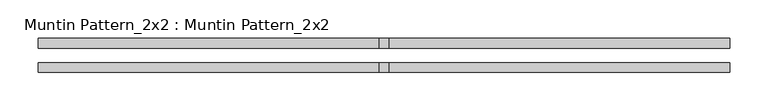
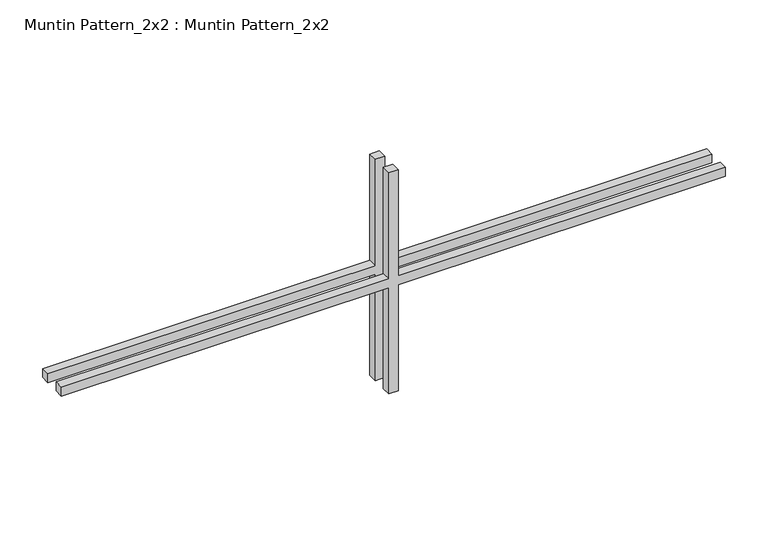
"""IFC4 building model written with IfcOpenShell, lengths in millimetres: proxy geometry, Muntin Pattern_2x2 : Muntin Pattern_2x2."""

from ifc_helpers import new_model, si_unit, frame, origin, place, context, project, spatial, polyline, outline, extrude, source, transform, mapped, element, save


def muntin_pattern_2x2_muntin_pattern_2x2_9ec9cf3e(model_context):
    return source(origin(), model_context, "Body", "SweptSolid", [
        extrude(outline(polyline([(165.0955927, -6.35), (165.0955927, -450.85), (152.3955927, -450.85), (152.3955927, -6.35), (0.0, -6.35), (0.0, 6.35), (152.3955927, 6.35), (152.3955927, 450.85), (165.0955927, 450.85), (165.0955927, 6.35), (317.4911855, 6.35), (317.4911855, -6.35), (165.0955927, -6.35)])), frame((0.0, 9.525, 0.0), z_axis=(0.0, 1.0, 0.0), x_axis=(0.0, 0.0, 1.0)), (0.0, 0.0, 1.0), 12.7),
        extrude(outline(polyline([(165.0955927, -6.35), (165.0955927, -450.85), (152.3955927, -450.85), (152.3955927, -6.35), (0.0, -6.35), (0.0, 6.35), (152.3955927, 6.35), (152.3955927, 450.85), (165.0955927, 450.85), (165.0955927, 6.35), (317.4911855, 6.35), (317.4911855, -6.35), (165.0955927, -6.35)])), frame((0.0, -22.225, 0.0), z_axis=(0.0, 1.0, 0.0), x_axis=(0.0, 0.0, 1.0)), (0.0, 0.0, 1.0), 12.7),
    ])


if __name__ == "__main__":
    model = new_model("IFC4")
    model_context = context("Model", 3, world=origin())
    ifc_project = project(units=[si_unit("LENGTHUNIT", "METRE", prefix="MILLI")], contexts=[model_context])
    site = spatial("IfcSite", under=ifc_project)
    building = spatial("IfcBuilding", under=site)
    placement = place(None, origin())
    muntin_pattern_2x2_muntin_pattern_2x2_shape = muntin_pattern_2x2_muntin_pattern_2x2_9ec9cf3e(model_context)
    element("IfcBuildingElementProxy", 1, Name="Muntin Pattern_2x2 : Muntin Pattern_2x2", ObjectType="Muntin Pattern_2x2 : Muntin Pattern_2x2", at=placement, inside=building, context=model_context, shape_type="MappedRepresentation", body=[
        mapped(muntin_pattern_2x2_muntin_pattern_2x2_shape, transform((0.0, 0.0, 0.0), x_axis=(1.0, 0.0, 0.0), y_axis=(0.0, 1.0, 0.0), z_axis=(0.0, 0.0, 1.0))),
    ])
    save(model, "model.ifc")

# Revit data of these elements
# Type "Muntin Pattern_2x2 : Muntin Pattern_2x2"
#   Width [instance default] = 4' - 0"
#   Thickness = 0' - 0 1/2"
#   Height [instance default] = 4' - 0"
#   Distance = 0' - 0 3/4"
#   Interior Material [instance default] = none
#   Exterior Material [instance default] = none
#   Default Elevation = 0
# Element 1 (IfcBuildingElementProxy, "Muntin Pattern_2x2 : Muntin Pattern_2x2")
#   Width = 2' - 11 1/2"
#   Height = 1' - 0.49965"
#   Interior Material = Wood - Stained
#   Exterior Material = Clad - White
#   Materials on its faces: "Clad - White", "Wood - Stained"
# Materials
#   "Clad - White": class "Wood", colour RGB 242 242 238, transparency 0, Cost = 0
#   "Wood - Stained": class "Wood", colour RGB 224 178 126, transparency 0, Cost = 0
